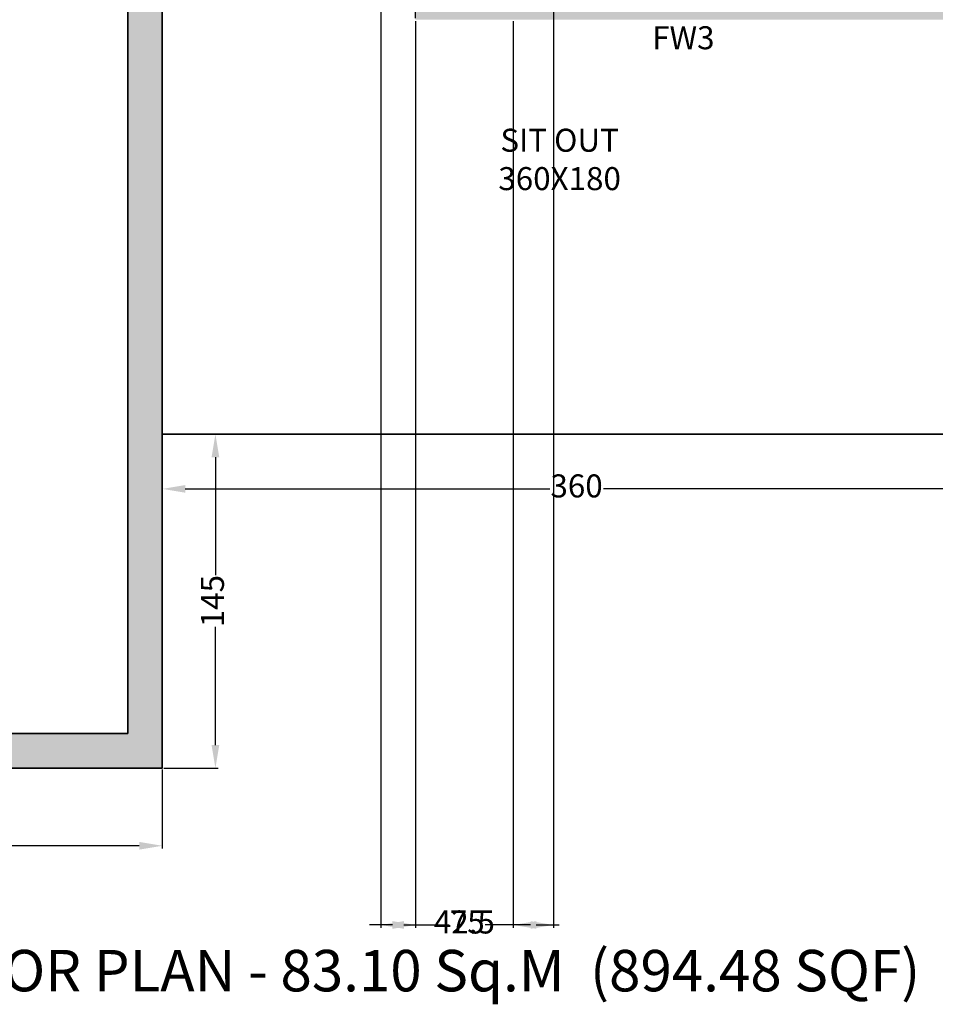
# Model space of a CAD drawing. Units: centimetres. Extents: x 2401 to 3632, y 2122 to 3526.
# Tile 3 of 10: x 2824 to 3221, y 2163 to 2591. Entities that reach past the tile are written whole.
import ezdxf

# ---------------------------------------------------------------- set-up
doc = ezdxf.new("R2010")
doc.units = ezdxf.units.CM
for name, color, linetype, lineweight in [('A-ANNO-DIMS', 9, 'Continuous', 18), ('A-ANNO-TEXT', 9, 'Continuous', 18), ('A-AREA-IDEN', 9, 'Continuous', 25), ('A-WALL', 7, 'Continuous', 35)]:
    doc.layers.add(name, color=color, linetype=linetype, lineweight=lineweight)
doc.layers.add('A-GLAZ-PATT', color=251, linetype='Continuous', lineweight=13, true_color=0x636466)
doc.layers.add('A-WALL-PATT', color=18, linetype='Continuous', lineweight=13, true_color=0x000000)
doc.styles.get("Standard").update_dxf_attribs({"font": 'arial.ttf'})
doc.dimstyles.new('ISO-25', dxfattribs={"dimtxt": 10, "dimasz": 10, "dimexe": 1.25, "dimexo": 0.625, "dimtad": 0, "dimtxsty": 'Standard', "dimcen": 2.5, "dimadec": 0, "dimazin": 0, "dimtfac": 1, "dimtmove": 0, "dimatfit": 3, "dimfxl": 1, "dimarcsym": 0})

# ---------------------------------------------------------------- blocks, each defined once
blk = doc.blocks.new('*D13')
at = {"layer": 'A-ANNO-DIMS', "color": 0, "lineweight": -2, "transparency": 16777216}
for p, q in [((2500.44, 2265.48), (2500.44, 2231.09)), ((2885.44, 2265.48), (2885.44, 2231.09)), ((2510.44, 2232.34), (2681.23, 2232.34)), ((2875.44, 2232.34), (2704.64, 2232.34))]:
    blk.add_line(p, q, dxfattribs=at)
at = {"layer": 'A-ANNO-DIMS', "color": 0, "transparency": 16777216}
for points in [[(2510.44, 2234.01), (2510.44, 2230.67), (2500.44, 2232.34)], [(2875.44, 2234.01), (2875.44, 2230.67), (2885.44, 2232.34)]]:
    blk.add_solid(points, dxfattribs=at)
at = {"layer": 'Defpoints', "color": 0, "transparency": 16777216}
for p in [(2500.44, 2266.1), (2885.44, 2266.1), (2885.44, 2232.34)]:
    blk.add_point(p, dxfattribs=at)
at = {"layer": 'A-ANNO-DIMS', "color": 0, "transparency": 16777216, "insert": (2692.94, 2232.34), "char_height": 10, "attachment_point": 5}
blk.add_mtext('385', dxfattribs=at)
blk = doc.blocks.new('*D15')
at = {"layer": 'A-ANNO-DIMS', "color": 0, "lineweight": -2, "transparency": 16777216}
for p, q in [((2885.44, 2410.48), (2885.44, 2386.08)), ((3245.44, 2410.48), (3245.44, 2386.08)), ((2895.44, 2387.33), (3053.78, 2387.33)), ((3235.44, 2387.33), (3077.09, 2387.33))]:
    blk.add_line(p, q, dxfattribs=at)
at = {"layer": 'A-ANNO-DIMS', "color": 0, "transparency": 16777216}
for points in [[(2895.44, 2389), (2895.44, 2385.67), (2885.44, 2387.33)], [(3235.44, 2389), (3235.44, 2385.67), (3245.44, 2387.33)]]:
    blk.add_solid(points, dxfattribs=at)
at = {"layer": 'Defpoints', "color": 0, "transparency": 16777216}
for p in [(2885.44, 2411.1), (3245.44, 2411.1), (3245.44, 2387.33)]:
    blk.add_point(p, dxfattribs=at)
at = {"layer": 'A-ANNO-DIMS', "color": 0, "transparency": 16777216, "insert": (3065.44, 2387.33), "char_height": 10, "attachment_point": 5}
blk.add_mtext('360', dxfattribs=at)
blk = doc.blocks.new('*D16')
at = {"layer": 'A-ANNO-DIMS', "color": 0, "lineweight": -2, "transparency": 16777216}
for p, q in [((2886.06, 2411.1), (2909.79, 2411.1)), ((2908.54, 2401.1), (2908.54, 2349.84)), ((2908.54, 2276.1), (2908.54, 2327.37)), ((2886.06, 2266.1), (2909.79, 2266.1))]:
    blk.add_line(p, q, dxfattribs=at)
at = {"layer": 'A-ANNO-DIMS', "color": 0, "transparency": 16777216}
for points in [[(2906.87, 2401.1), (2910.21, 2401.1), (2908.54, 2411.1)], [(2906.87, 2276.1), (2910.21, 2276.1), (2908.54, 2266.1)]]:
    blk.add_solid(points, dxfattribs=at)
at = {"layer": 'Defpoints', "color": 0, "transparency": 16777216}
for p in [(2885.44, 2411.1), (2885.44, 2266.1), (2908.54, 2266.1)]:
    blk.add_point(p, dxfattribs=at)
at = {"layer": 'A-ANNO-DIMS', "color": 0, "transparency": 16777216, "insert": (2908.54, 2338.6), "char_height": 10, "attachment_point": 5, "rotation": 90}
blk.add_mtext('145', dxfattribs=at)
blk = doc.blocks.new('*D47')
at = {"layer": 'A-ANNO-DIMS', "color": 0, "lineweight": -2, "transparency": 16777216}
for p, q in [((2995.44, 2590.48), (2995.44, 2196.7)), ((3037.94, 2590.48), (3037.94, 2196.7)), ((2985.44, 2197.95), (2975.44, 2197.95)), ((2995.44, 2197.95), (3002.83, 2197.95)), ((3037.94, 2197.95), (3030.54, 2197.95)), ((3047.94, 2197.95), (3057.94, 2197.95))]:
    blk.add_line(p, q, dxfattribs=at)
at = {"layer": 'A-ANNO-DIMS', "color": 0, "transparency": 16777216}
for points in [[(2985.44, 2199.62), (2985.44, 2196.29), (2995.44, 2197.95)], [(3047.94, 2199.62), (3047.94, 2196.29), (3037.94, 2197.95)]]:
    blk.add_solid(points, dxfattribs=at)
at = {"layer": 'Defpoints', "color": 0, "transparency": 16777216}
for p in [(2995.44, 2591.1), (3037.94, 2591.1), (2995.44, 2197.95)]:
    blk.add_point(p, dxfattribs=at)
at = {"layer": 'A-ANNO-DIMS', "color": 0, "transparency": 16777216, "insert": (3016.69, 2197.95), "char_height": 10, "attachment_point": 5}
blk.add_mtext('42.5', dxfattribs=at)
blk = doc.blocks.new('*D50')
at = {"layer": 'A-ANNO-DIMS', "color": 0, "lineweight": -2, "transparency": 16777216}
for p, q in [((2980.44, 3095.48), (2980.44, 2196.7)), ((3055.44, 3080.48), (3055.44, 2196.7)), ((2990.44, 2197.95), (3010.15, 2197.95)), ((3045.44, 2197.95), (3025.72, 2197.95))]:
    blk.add_line(p, q, dxfattribs=at)
at = {"layer": 'A-ANNO-DIMS', "color": 0, "transparency": 16777216}
for points in [[(2990.44, 2199.62), (2990.44, 2196.29), (2980.44, 2197.95)], [(3045.44, 2199.62), (3045.44, 2196.29), (3055.44, 2197.95)]]:
    blk.add_solid(points, dxfattribs=at)
at = {"layer": 'Defpoints', "color": 0, "transparency": 16777216}
for p in [(2980.44, 3096.1), (3055.44, 3081.1), (3055.44, 2197.95)]:
    blk.add_point(p, dxfattribs=at)
at = {"layer": 'A-ANNO-DIMS', "color": 0, "transparency": 16777216, "insert": (3017.94, 2197.95), "char_height": 10, "attachment_point": 5}
blk.add_mtext('75', dxfattribs=at)
blk = doc.blocks.new('*D52')
at = {"layer": 'A-ANNO-DIMS', "color": 0, "lineweight": -2, "transparency": 16777216}
for p, q in [((2885.44, 2411.73), (2885.44, 3520.5)), ((2895.44, 3519.25), (2929.25, 3519.25)), ((2985.44, 3519.25), (2951.62, 3519.25)), ((2995.44, 2591.73), (2995.44, 3520.5))]:
    blk.add_line(p, q, dxfattribs=at)
at = {"layer": 'A-ANNO-DIMS', "color": 0, "transparency": 16777216}
for points in [[(2895.44, 3520.92), (2895.44, 3517.59), (2885.44, 3519.25)], [(2985.44, 3520.92), (2985.44, 3517.59), (2995.44, 3519.25)]]:
    blk.add_solid(points, dxfattribs=at)
at = {"layer": 'Defpoints', "color": 0, "transparency": 16777216}
for p in [(2995.44, 3519.25), (2995.44, 2591.1), (2885.44, 2411.1)]:
    blk.add_point(p, dxfattribs=at)
at = {"layer": 'A-ANNO-DIMS', "color": 0, "transparency": 16777216, "insert": (2940.44, 3519.25), "char_height": 10, "attachment_point": 5}
blk.add_mtext('110', dxfattribs=at)

msp = doc.modelspace()

# ---------------------------------------------------------------- hatches: boundary and pattern name
at = {"layer": 'A-GLAZ-PATT'}
h = msp.add_hatch(color=256, dxfattribs=at)
h.dxf.hatch_style = 1
h.paths.add_polyline_path([(2505.936, 3356.104), (2500.436, 3356.104), (2500.436, 3301.104), (2505.936, 3301.104)])
h.paths.add_polyline_path([(2509.936, 3356.104), (2505.936, 3356.104), (2505.936, 3301.104), (2509.936, 3301.104)])
h.paths.add_polyline_path([(2515.436, 3335.674), (2515.436, 3356.104), (2509.936, 3356.104), (2509.936, 3301.104), (2515.436, 3301.104)])
h.paths.add_polyline_path([(2509.936, 3301.104), (2505.936, 3301.104), (2505.936, 3261.104), (2509.936, 3261.104)])
h.paths.add_polyline_path([(2515.436, 3301.104), (2509.936, 3301.104), (2509.936, 3261.104), (2515.436, 3261.104)])
h.paths.add_polyline_path([(2505.936, 3301.104), (2500.436, 3301.104), (2500.436, 3261.104), (2505.936, 3261.104)])
h.paths.add_polyline_path([(2515.436, 3261.104), (2509.936, 3261.104), (2509.936, 3206.104), (2515.436, 3206.104)])
h.paths.add_polyline_path([(2505.936, 3261.104), (2500.436, 3261.104), (2500.436, 3206.104), (2505.936, 3206.104)])
h.paths.add_polyline_path([(2509.936, 3261.104), (2505.936, 3261.104), (2505.936, 3206.104), (2509.936, 3206.104)])
h.paths.add_polyline_path([(3127.936, 3451.104), (3072.936, 3451.104), (3072.936, 3445.604), (3127.936, 3445.604)])
h.paths.add_polyline_path([(3032.936, 3441.604), (2977.936, 3441.604), (2977.936, 3436.104), (3032.936, 3436.104)])
h.paths.add_polyline_path([(3032.936, 3451.104), (2977.936, 3451.104), (2977.936, 3445.604), (3032.936, 3445.604)])
h.paths.add_polyline_path([(3032.936, 3445.604), (2977.936, 3445.604), (2977.936, 3441.604), (3032.936, 3441.604)])
h.paths.add_polyline_path([(3072.936, 3451.104), (3032.936, 3451.104), (3032.936, 3445.604), (3072.936, 3445.604)])
h.paths.add_polyline_path([(3072.936, 3445.604), (3032.936, 3445.604), (3032.936, 3441.604), (3072.936, 3441.604)])
h.paths.add_polyline_path([(3072.936, 3441.604), (3032.936, 3441.604), (3032.936, 3436.104), (3072.936, 3436.104)])
h.paths.add_polyline_path([(3127.936, 3441.604), (3072.936, 3441.604), (3072.936, 3436.104), (3127.936, 3436.104)])
h.paths.add_polyline_path([(3127.936, 3445.604), (3072.936, 3445.604), (3072.936, 3441.604), (3127.936, 3441.604)])
h.paths.add_polyline_path([(3245.436, 3356.104), (3239.936, 3356.104), (3239.936, 3301.104), (3245.436, 3301.104)])
h.paths.add_polyline_path([(3239.936, 3356.104), (3235.936, 3356.104), (3235.936, 3301.104), (3239.936, 3301.104)])
h.paths.add_polyline_path([(3235.936, 3356.104), (3230.436, 3356.104), (3230.436, 3301.104), (3235.936, 3301.104)])
h.paths.add_polyline_path([(3235.936, 3301.104), (3230.436, 3301.104), (3230.436, 3261.104), (3235.936, 3261.104)])
h.paths.add_polyline_path([(3239.936, 3301.104), (3235.936, 3301.104), (3235.936, 3261.104), (3239.936, 3261.104)])
h.paths.add_polyline_path([(3245.436, 3301.104), (3239.936, 3301.104), (3239.936, 3261.104), (3245.436, 3261.104)])
h.paths.add_polyline_path([(3245.436, 3261.104), (3239.936, 3261.104), (3239.936, 3206.104), (3245.436, 3206.104)])
h.paths.add_polyline_path([(3239.936, 3261.104), (3235.936, 3261.104), (3235.936, 3206.104), (3239.936, 3206.104)])
h.paths.add_polyline_path([(3235.936, 3261.104), (3230.436, 3261.104), (3230.436, 3206.104), (3235.936, 3206.104)])
h.paths.add_polyline_path([(3239.936, 3036.104), (3235.936, 3036.104), (3235.936, 2976.104), (3239.936, 2976.104)])
h.paths.add_polyline_path([(3235.936, 3036.104), (3230.436, 3036.104), (3230.436, 2976.104), (3235.936, 2976.104)])
h.paths.add_polyline_path([(3245.436, 3036.104), (3239.936, 3036.104), (3239.936, 2976.104), (3245.436, 2976.104)])
h.paths.add_polyline_path([(3235.936, 2836.104), (3230.436, 2836.104), (3230.436, 2781.104), (3235.936, 2781.104)])
h.paths.add_polyline_path([(3245.436, 2836.104), (3239.936, 2836.104), (3239.936, 2781.104), (3245.436, 2781.104)])
h.paths.add_polyline_path([(3239.936, 2836.104), (3235.936, 2836.104), (3235.936, 2781.104), (3239.936, 2781.104)])
h.paths.add_polyline_path([(3245.436, 2781.104), (3239.936, 2781.104), (3239.936, 2741.104), (3245.436, 2741.104)])
h.paths.add_polyline_path([(3239.936, 2781.104), (3235.936, 2781.104), (3235.936, 2741.104), (3239.936, 2741.104)])
h.paths.add_polyline_path([(3235.936, 2781.104), (3230.436, 2781.104), (3230.436, 2741.104), (3235.936, 2741.104)])
h.paths.add_polyline_path([(3245.436, 2741.104), (3239.936, 2741.104), (3239.936, 2686.104), (3245.436, 2686.104)])
h.paths.add_polyline_path([(3239.936, 2741.104), (3235.936, 2741.104), (3235.936, 2686.104), (3239.936, 2686.104)])
h.paths.add_polyline_path([(3235.936, 2741.104), (3230.436, 2741.104), (3230.436, 2686.104), (3235.936, 2686.104)])
h.paths.add_polyline_path([(3187.936, 2606.104), (3132.936, 2606.104), (3132.936, 2600.604), (3187.936, 2600.604)])
h.paths.add_polyline_path([(3187.936, 2600.604), (3132.936, 2600.604), (3132.936, 2596.604), (3187.936, 2596.604)])
h.paths.add_polyline_path([(3187.936, 2596.604), (3132.936, 2596.604), (3132.936, 2591.104), (3187.936, 2591.104)])
h.paths.add_polyline_path([(3132.936, 2596.604), (3092.936, 2596.604), (3092.936, 2591.104), (3132.936, 2591.104)])
h.paths.add_polyline_path([(3132.936, 2600.604), (3092.936, 2600.604), (3092.936, 2596.604), (3132.936, 2596.604)])
h.paths.add_polyline_path([(3132.936, 2606.104), (3092.936, 2606.104), (3092.936, 2600.604), (3132.936, 2600.604)])
h.paths.add_polyline_path([(3092.936, 2596.604), (3037.936, 2596.604), (3037.936, 2591.104), (3092.936, 2591.104)])
h.paths.add_polyline_path([(3092.936, 2600.604), (3037.936, 2600.604), (3037.936, 2596.604), (3092.936, 2596.604)])
h.paths.add_polyline_path([(3092.936, 2606.104), (3037.936, 2606.104), (3037.936, 2600.604), (3092.936, 2600.604)])
h.paths.add_polyline_path([(2803.613, 3432.66), (2826.471, 3432.66), (2826.471, 3453.267), (2803.613, 3453.267)], flags=9)
h.paths.add_polyline_path([(2904.038, 3087.418), (2926.896, 3087.418), (2926.896, 3108.025), (2904.038, 3108.025)], flags=9)
h.paths.add_polyline_path([(2801.908, 3105.391), (2824.766, 3105.391), (2824.766, 3125.998), (2801.908, 3125.998)], flags=9)
h.paths.add_polyline_path([(2757.576, 2660.284), (2780.434, 2660.284), (2780.434, 2680.892), (2757.576, 2680.892)], flags=9)
h.paths.add_polyline_path([(3004.446, 3080.825), (3027.304, 3080.825), (3027.304, 3101.432), (3004.446, 3101.432)], flags=9)
h.paths.add_polyline_path([(2805.63, 2777.019), (2828.489, 2777.019), (2828.489, 2797.626), (2805.63, 2797.626)], flags=9)
h.paths.add_polyline_path([(3094.334, 2572.754), (3128.823, 2572.754), (3128.823, 2593.361), (3094.334, 2593.361)], flags=9)
h.paths.add_polyline_path([(2931.792, 2588.154), (2946.88, 2588.154), (2946.88, 2608.761), (2931.792, 2608.761)], flags=9)
h.paths.add_polyline_path([(2582.951, 2415.87), (2664.015, 2415.87), (2664.015, 2453.184), (2582.951, 2453.184)], flags=9)
h.paths.add_polyline_path([(2622.234, 2685.113), (2683.168, 2685.113), (2683.168, 2722.427), (2622.234, 2722.427)], flags=9)
h.paths.add_polyline_path([(3027.646, 2511.408), (3088.58, 2511.408), (3088.58, 2548.722), (3027.646, 2548.722)], flags=9)
h.paths.add_polyline_path([(3020.004, 2720.966), (3092.521, 2720.966), (3092.521, 2758.281), (3020.004, 2758.281)], flags=9)
h.paths.add_polyline_path([(2628.506, 2930.416), (2689.441, 2930.416), (2689.441, 2967.73), (2628.506, 2967.73)], flags=9)
h.paths.add_polyline_path([(3056.573, 2986.666), (3117.507, 2986.666), (3117.507, 3023.981), (3056.573, 3023.981)], flags=9)
h.paths.add_polyline_path([(3083.425, 3281.357), (3164.489, 3281.357), (3164.489, 3318.672), (3083.425, 3318.672)], flags=9)
h.paths.add_polyline_path([(2658.367, 3249.15), (2724.683, 3249.15), (2724.683, 3286.465), (2658.367, 3286.465)], flags=9)
at = {"layer": 'A-WALL-PATT'}
h = msp.add_hatch(color=256, dxfattribs=at)
h.dxf.hatch_style = 1
h.paths.add_polyline_path([(2765.436, 3451.104), (2500.436, 3451.104), (2500.436, 3356.104), (2515.436, 3356.104), (2515.436, 3436.104), (2765.436, 3436.104)])
h.paths.add_polyline_path([(3245.436, 3451.104), (3127.936, 3451.104), (3127.936, 3436.104), (3185.226, 3436.104), (3185.226, 3436.735), (3230.436, 3436.735), (3230.436, 3356.104), (3245.436, 3356.104)])
h.paths.add_polyline_path([(3245.436, 2686.104), (3230.436, 2686.104), (3230.436, 2606.104), (3187.936, 2606.104), (3187.936, 2591.104), (3245.436, 2591.104)])
h.paths.add_polyline_path([(3037.936, 2606.104), (2995.436, 2606.104), (2995.436, 2591.104), (3037.936, 2591.104)])
h.paths.add_polyline_path([(3245.436, 2976.104), (3230.436, 2976.104), (3230.436, 2931.104), (2980.436, 2931.104), (2980.436, 3096.104), (2965.436, 3096.104), (2965.436, 2916.104), (3230.436, 2916.104), (3230.436, 2836.104), (3245.436, 2836.104)])
h.paths.add_polyline_path([(3230.436, 3096.104), (3055.436, 3096.104), (3055.436, 3081.104), (3230.436, 3081.104)], flags=17)
h.paths.add_polyline_path([(2977.936, 3451.104), (2860.436, 3451.104), (2860.436, 3096.104), (2875.436, 3096.104), (2875.436, 3436.104), (2977.936, 3436.104)])
h.paths.add_polyline_path([(2765.436, 3126.104), (2515.436, 3126.104), (2515.436, 3206.104), (2500.436, 3206.104), (2500.436, 3028.604), (2515.436, 3028.604), (2515.436, 3111.104), (2765.436, 3111.104)])
h.paths.add_polyline_path([(2780.436, 2796.104), (2515.436, 2796.104), (2515.436, 2878.604), (2500.436, 2878.604), (2500.436, 2736.104), (2515.436, 2736.104), (2515.436, 2781.104), (2765.436, 2781.104), (2765.436, 2706.104), (2780.436, 2706.104)])
h.paths.add_polyline_path([(2780.436, 2631.104), (2515.436, 2631.104), (2515.436, 2676.104), (2500.436, 2676.104), (2500.436, 2523.604), (2515.436, 2523.604), (2515.436, 2616.104), (2780.436, 2616.104)])
h.paths.add_polyline_path([(2885.436, 2796.104), (2870.436, 2796.104), (2870.436, 2281.104), (2762.936, 2281.104), (2762.936, 2266.104), (2885.436, 2266.104)])
h.paths.add_polyline_path([(2612.936, 2281.104), (2515.436, 2281.104), (2515.436, 2373.604), (2500.436, 2373.604), (2500.436, 2266.104), (2612.936, 2266.104)])

# ---------------------------------------------------------------- linework, layer by layer
at = {"layer": 'A-WALL'}
for p in [(2870.436, 2796.104), (2515.436, 2281.104)]:
    msp.add_line(p, (2870.436, 2281.104), dxfattribs=at)
for points in [[(2765.436, 3451.104), (2500.436, 3451.104), (2500.436, 2266.104), (2885.436, 2266.104), (2885.436, 2796.104)], [(2885.436, 2411.104), (3245.436, 2411.104), (3245.436, 3451.104), (2860.436, 3451.104)]]:
    msp.add_lwpolyline(points, dxfattribs=at)

# ---------------------------------------------------------------- texts
at = {"layer": 'A-ANNO-TEXT', "attachment_point": 1}
for s, width, insert, char_height in [('\\pxqc;FW3', 66.28614, (3078.691, 2588.255), 10), ('\\pxqc;{\\fCalifornian FB|b1|i0|c0|p18;GROUND FLOOR PLAN - 83.10 Sq.M  (894.48 SQF)}', 622.58197, (2627.432, 2187.118), 18)]:
    msp.add_mtext_dynamic_manual_height_columns(s, width=width, gutter_width=12.5, heights=[0], dxfattribs=dict(at, insert=insert, char_height=char_height))
at = {"layer": 'A-AREA-IDEN', "insert": (3024.929, 2543.753), "char_height": 10, "attachment_point": 1}
msp.add_mtext_dynamic_manual_height_columns('\\pxqc;SIT OUT\\P360X180', width=66.28614, gutter_width=12.5, heights=[0], dxfattribs=at)

# ---------------------------------------------------------------- dimensions: what is measured, and where the dimension line sits
at = {"layer": 'A-ANNO-DIMS'}
for base, p1, p2, override, picture, middle in [((2995.436, 3519.254), (2885.436, 2411.104), (2995.436, 2591.104), {"dimdec": 0, "dimlfac": 1, "dimrnd": 0, "dimzin": 0, "dimdsep": 46, "dimlunit": 2}, '*D52', (2940.436, 3519.254)), ((3055.436, 2197.954), (2980.436, 3096.104), (3055.436, 3081.104), {"dimdec": 0, "dimlfac": 1, "dimrnd": 0, "dimzin": 0, "dimdsep": 46, "dimlunit": 2}, '*D50', (3017.936, 2197.954)), ((2995.436, 2197.954), (3037.936, 2591.104), (2995.436, 2591.104), {"dimdec": 1, "dimlfac": 1, "dimrnd": 0, "dimzin": 0, "dimdsep": 46, "dimlunit": 2}, '*D47', (3016.686, 2197.954)), ((3245.436, 2387.332), (2885.436, 2411.104), (3245.436, 2411.104), {"dimclrd": 0, "dimclre": 0, "dimclrt": 0}, '*D15', (3065.436, 2387.332)), ((2885.436, 2232.34), (2500.436, 2266.104), (2885.436, 2266.104), {"dimclrd": 0, "dimclre": 0, "dimclrt": 0}, '*D13', (2692.936, 2232.34))]:
    dim = msp.add_linear_dim(base=base, p1=p1, p2=p2, dimstyle='ISO-25', override=override, dxfattribs=at)
    dim.commit()
    dim.dimension.update_dxf_attribs({"geometry": picture, "text_midpoint": middle})
dim = msp.add_linear_dim(base=(2908.54, 2266.104), p1=(2885.436, 2411.104), p2=(2885.436, 2266.104), angle=90, dimstyle='ISO-25', override={"dimclrd": 0, "dimclre": 0, "dimclrt": 0}, dxfattribs=at)
dim.commit()
dim.dimension.update_dxf_attribs({"geometry": '*D16', "text_midpoint": (2908.54, 2338.604)})

doc.saveas('drawing.dxf')
